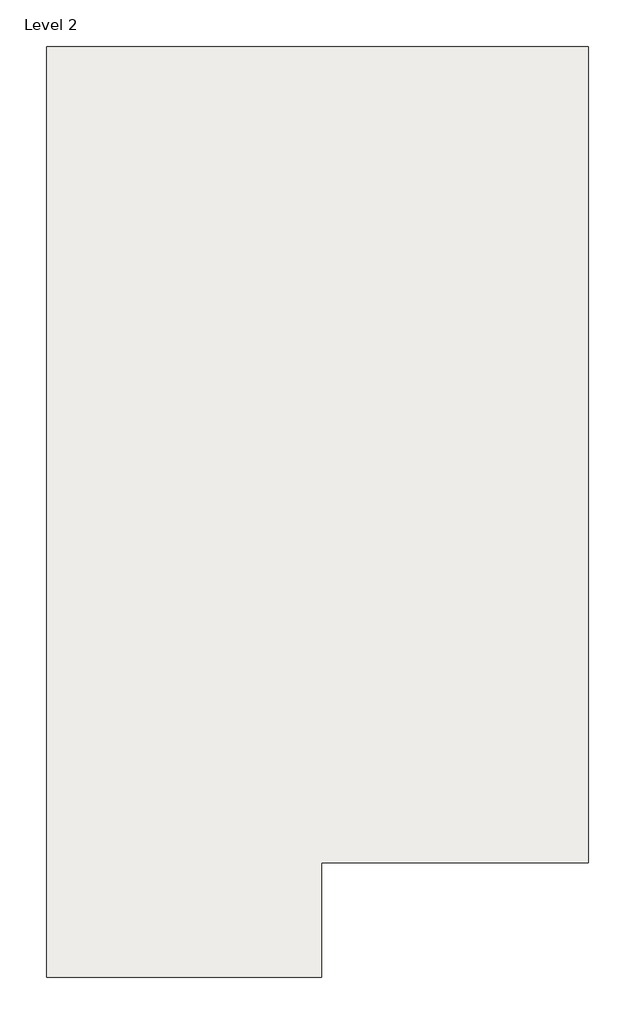
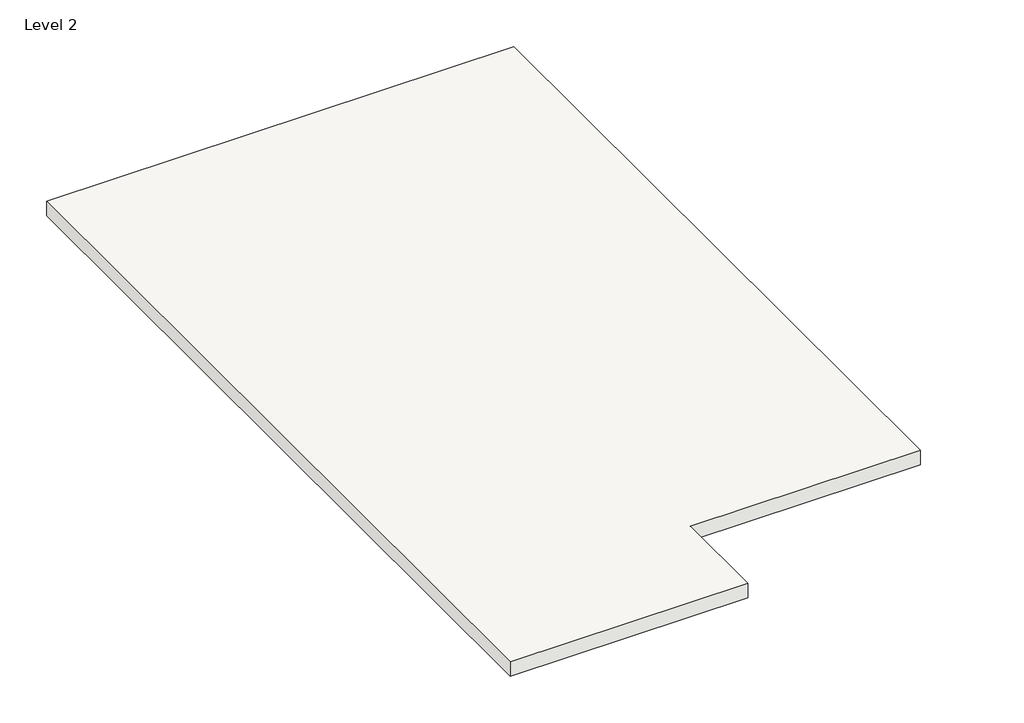
# One storey: 1 roof.
"""IFC4 building model written with IfcOpenShell, lengths in millimetres."""

from ifc_helpers import new_model, si_unit, frame, origin, place, context, project, spatial, polyline, outline, extrude, element, save

model = new_model("IFC4")

# Units and contexts
model_context = context("Model", 3, world=origin())
ifc_project = project(units=[si_unit("LENGTHUNIT", "METRE", prefix="MILLI")], contexts=[model_context])

# Site, building, storey
site = spatial("IfcSite", under=ifc_project)
building = spatial("IfcBuilding", under=site)
storey = spatial("IfcBuildingStorey", under=building, Name="Level 2", Elevation=3048.0)

# Roof
placement = place(None, origin())
element("IfcRoof", 1, ObjectType="Generic - 12\"", at=placement, inside=storey, context=model_context, shape_type="SweptSolid", body=[
    extrude(outline(polyline([(-12245.0060487, 9424.1432954), (-2897.8060487, 9424.1432954), (-2897.8060487, -4647.4567046), (-7495.2060487, -4647.4567046), (-7495.2060487, -6628.6567046), (-12245.0060487, -6628.6567046), (-12245.0060487, 9424.1432954)])), frame((0.0, 0.0, 3048.0), z_axis=(0.0, 0.0, 1.0), x_axis=(1.0, 0.0, 0.0)), (0.0, 0.0, 1.0), 304.8),
])

save(model, "model.ifc")

# Revit data of these elements
# Type "Generic - 12\""
#   Assembly Code = "B1020"
#   Layers, outside or top first: 1' - 0" "Brick, Soldier Course" (function 1)
# Element 1 (IfcRoof, "Generic - 12\"")
#   built-in parameter 1001705 = 11 (stored number, unit not read)
#   built-in parameter 1001710 = 33615
#   Phase Created = New Construction
#   Materials on its faces: "Brick, Soldier Course"
# Materials
#   "Brick, Soldier Course": class "Masonry", colour RGB 170 98 104, transparency 0, Description = "Common brick soldier coursed", Cost = 0
